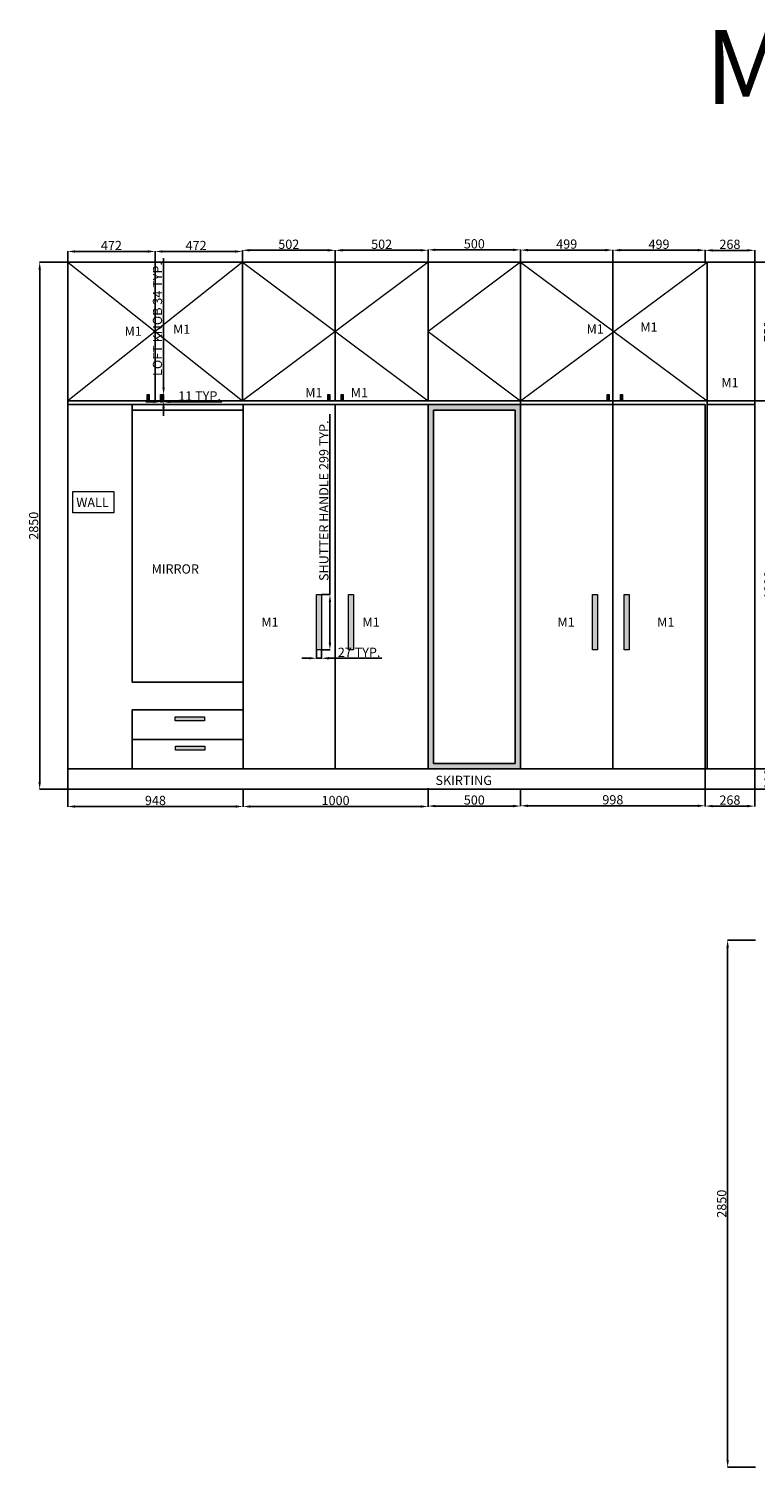
# Model space of a CAD drawing. Units: millimetres. Extents: x 46070 to 59439, y 6883 to 14761.
# Tile 1 of 5: x 46070 to 49997, y 6983 to 14761. Entities that reach past the tile are written whole.
import ezdxf

# ---------------------------------------------------------------- set-up
doc = ezdxf.new("R2010")
doc.units = ezdxf.units.MM
for name, color, linetype, lineweight in [('A-ANNO-DIMS', 2, 'Continuous', 18), ('A-ANNO-TEXT', 7, 'Continuous', 18), ('A-ELEV', 7, 'Continuous', 25), ('A-ELEV-OPEN', 1, 'Continuous', 13), ('A-ELEV-PATT', 8, 'Continuous', 13), ('A-FURN-HDWR', 4, 'Continuous', 18)]:
    doc.layers.add(name, color=color, linetype=linetype, lineweight=lineweight)
doc.styles.get("Standard").update_dxf_attribs({"font": 'arial.ttf'})
doc.dimstyles.new('ISO-25', dxfattribs={"dimtxt": 50, "dimasz": 40, "dimexe": 1.25, "dimexo": 0.625, "dimtad": 1, "dimtxsty": 'Standard', "dimcen": 2.5, "dimadec": 0, "dimazin": 0, "dimtfac": 1, "dimtmove": 0, "dimatfit": 3, "dimfxl": 1, "dimarcsym": 0})

# ---------------------------------------------------------------- blocks, each defined once
blk = doc.blocks.new('*D1')
at = {"layer": 'A-ANNO-DIMS', "color": 0, "lineweight": -2, "transparency": 16777216}
for p, q in [((49995.3, 10759), (50105.5, 10759)), ((50104.2, 10689), (50104.2, 10719)), ((49995.3, 10649), (50105.5, 10649))]:
    blk.add_line(p, q, dxfattribs=at)
at = {"layer": 'A-ANNO-DIMS', "color": 0, "transparency": 16777216}
for points in [[(50097.5, 10719), (50110.9, 10719), (50104.2, 10759)], [(50097.5, 10689), (50110.9, 10689), (50104.2, 10649)]]:
    blk.add_solid(points, dxfattribs=at)
at = {"layer": 'Defpoints', "color": 0, "transparency": 16777216}
for p in [(49994.7, 10759), (50104.2, 10759), (49994.7, 10649)]:
    blk.add_point(p, dxfattribs=at)
at = {"layer": 'A-ANNO-DIMS', "color": 0, "transparency": 16777216, "insert": (50078.1, 10703.9), "char_height": 50, "attachment_point": 5, "rotation": 90}
blk.add_mtext('110', dxfattribs=at)
blk = doc.blocks.new('*D2')
at = {"layer": 'A-ANNO-DIMS', "color": 0, "lineweight": -2, "transparency": 16777216}
for p, q in [((49995.3, 12749), (50105.3, 12749)), ((50104.1, 10799), (50104.1, 12709)), ((49995.3, 10759), (50105.3, 10759))]:
    blk.add_line(p, q, dxfattribs=at)
at = {"layer": 'A-ANNO-DIMS', "color": 0, "transparency": 16777216}
for points in [[(50097.4, 12709), (50110.8, 12709), (50104.1, 12749)], [(50097.4, 10799), (50110.8, 10799), (50104.1, 10759)]]:
    blk.add_solid(points, dxfattribs=at)
at = {"layer": 'Defpoints', "color": 0, "transparency": 16777216}
for p in [(49994.7, 12749), (50104.1, 12749), (49994.7, 10759)]:
    blk.add_point(p, dxfattribs=at)
at = {"layer": 'A-ANNO-DIMS', "color": 0, "transparency": 16777216, "insert": (50077.9, 11754), "char_height": 50, "attachment_point": 5, "rotation": 90}
blk.add_mtext('1990', dxfattribs=at)
blk = doc.blocks.new('*D3')
at = {"layer": 'A-ANNO-DIMS', "color": 0, "lineweight": -2, "transparency": 16777216}
for p, q in [((49995.3, 13499), (50103.6, 13499)), ((50102.3, 12789), (50102.3, 13459)), ((49995.3, 12749), (50103.6, 12749))]:
    blk.add_line(p, q, dxfattribs=at)
at = {"layer": 'A-ANNO-DIMS', "color": 0, "transparency": 16777216}
for points in [[(50095.6, 13459), (50109, 13459), (50102.3, 13499)], [(50095.6, 12789), (50109, 12789), (50102.3, 12749)]]:
    blk.add_solid(points, dxfattribs=at)
at = {"layer": 'Defpoints', "color": 0, "transparency": 16777216}
for p in [(49994.7, 13499), (50102.3, 13499), (49994.7, 12749)]:
    blk.add_point(p, dxfattribs=at)
at = {"layer": 'A-ANNO-DIMS', "color": 0, "transparency": 16777216, "insert": (50076.2, 13124), "char_height": 50, "attachment_point": 5, "rotation": 90}
blk.add_mtext('750', dxfattribs=at)
blk = doc.blocks.new('*D4')
at = {"layer": 'A-ANNO-DIMS', "color": 0, "lineweight": -2, "transparency": 16777216}
for p, q in [((48728.7, 13499.7), (48728.7, 13565.8)), ((49187.7, 13564.6), (48768.7, 13564.6)), ((49227.7, 13499.7), (49227.7, 13565.8))]:
    blk.add_line(p, q, dxfattribs=at)
at = {"layer": 'A-ANNO-DIMS', "color": 0, "transparency": 16777216}
for points in [[(48768.7, 13571.2), (48768.7, 13557.9), (48728.7, 13564.6)], [(49187.7, 13571.2), (49187.7, 13557.9), (49227.7, 13564.6)]]:
    blk.add_solid(points, dxfattribs=at)
at = {"layer": 'Defpoints', "color": 0, "transparency": 16777216}
for p in [(48728.7, 13564.6), (48728.7, 13499), (49227.7, 13499)]:
    blk.add_point(p, dxfattribs=at)
at = {"layer": 'A-ANNO-DIMS', "color": 0, "transparency": 16777216, "insert": (48978.2, 13590.7), "char_height": 50, "attachment_point": 5}
blk.add_mtext('499', dxfattribs=at)
blk = doc.blocks.new('*D5')
at = {"layer": 'A-ANNO-DIMS', "color": 0, "lineweight": -2, "transparency": 16777216}
for p, q in [((49227.7, 13499.7), (49227.7, 13565.1)), ((49267.7, 13563.9), (49686.7, 13563.9)), ((49726.7, 13499.7), (49726.7, 13565.1))]:
    blk.add_line(p, q, dxfattribs=at)
at = {"layer": 'A-ANNO-DIMS', "color": 0, "transparency": 16777216}
for points in [[(49267.7, 13570.6), (49267.7, 13557.2), (49227.7, 13563.9)], [(49686.7, 13570.6), (49686.7, 13557.2), (49726.7, 13563.9)]]:
    blk.add_solid(points, dxfattribs=at)
at = {"layer": 'Defpoints', "color": 0, "transparency": 16777216}
for p in [(49726.7, 13563.9), (49227.7, 13499), (49726.7, 13499)]:
    blk.add_point(p, dxfattribs=at)
at = {"layer": 'A-ANNO-DIMS', "color": 0, "transparency": 16777216, "insert": (49477.2, 13590), "char_height": 50, "attachment_point": 5}
blk.add_mtext('499', dxfattribs=at)
blk = doc.blocks.new('*D6')
at = {"layer": 'A-ANNO-DIMS', "color": 0, "lineweight": -2, "transparency": 16777216}
for p, q in [((48728.7, 10648.4), (48728.7, 10558.4)), ((49726.7, 10648.4), (49726.7, 10558.4)), ((49686.7, 10559.6), (48768.7, 10559.6))]:
    blk.add_line(p, q, dxfattribs=at)
at = {"layer": 'A-ANNO-DIMS', "color": 0, "transparency": 16777216}
for points in [[(48768.7, 10566.3), (48768.7, 10552.9), (48728.7, 10559.6)], [(49686.7, 10566.3), (49686.7, 10552.9), (49726.7, 10559.6)]]:
    blk.add_solid(points, dxfattribs=at)
at = {"layer": 'Defpoints', "color": 0, "transparency": 16777216}
for p in [(48728.7, 10649), (49726.7, 10649), (48728.7, 10559.6)]:
    blk.add_point(p, dxfattribs=at)
at = {"layer": 'A-ANNO-DIMS', "color": 0, "transparency": 16777216, "insert": (49227.7, 10585.8), "char_height": 50, "attachment_point": 5}
blk.add_mtext('998', dxfattribs=at)
blk = doc.blocks.new('*D7')
at = {"layer": 'A-ANNO-DIMS', "color": 0, "lineweight": -2, "transparency": 16777216}
for p, q in [((48228.7, 10648.4), (48228.7, 10557.1)), ((48728.7, 10648.4), (48728.7, 10557.1)), ((48268.7, 10558.4), (48688.7, 10558.4))]:
    blk.add_line(p, q, dxfattribs=at)
at = {"layer": 'A-ANNO-DIMS', "color": 0, "transparency": 16777216}
for points in [[(48268.7, 10565), (48268.7, 10551.7), (48228.7, 10558.4)], [(48688.7, 10565), (48688.7, 10551.7), (48728.7, 10558.4)]]:
    blk.add_solid(points, dxfattribs=at)
at = {"layer": 'Defpoints', "color": 0, "transparency": 16777216}
for p in [(48228.7, 10649), (48728.7, 10649), (48728.7, 10558.4)]:
    blk.add_point(p, dxfattribs=at)
at = {"layer": 'A-ANNO-DIMS', "color": 0, "transparency": 16777216, "insert": (48478.7, 10584.5), "char_height": 50, "attachment_point": 5}
blk.add_mtext('500', dxfattribs=at)
blk = doc.blocks.new('*D8')
at = {"layer": 'A-ANNO-DIMS', "color": 0, "lineweight": -2, "transparency": 16777216}
for p, q in [((48228.7, 13499.7), (48228.7, 13567.1)), ((48268.7, 13565.8), (48688.7, 13565.8)), ((48728.7, 13499.7), (48728.7, 13567.1))]:
    blk.add_line(p, q, dxfattribs=at)
at = {"layer": 'A-ANNO-DIMS', "color": 0, "transparency": 16777216}
for points in [[(48268.7, 13572.5), (48268.7, 13559.2), (48228.7, 13565.8)], [(48688.7, 13572.5), (48688.7, 13559.2), (48728.7, 13565.8)]]:
    blk.add_solid(points, dxfattribs=at)
at = {"layer": 'Defpoints', "color": 0, "transparency": 16777216}
for p in [(48728.7, 13565.8), (48228.7, 13499), (48728.7, 13499)]:
    blk.add_point(p, dxfattribs=at)
at = {"layer": 'A-ANNO-DIMS', "color": 0, "transparency": 16777216, "insert": (48478.7, 13592), "char_height": 50, "attachment_point": 5}
blk.add_mtext('500', dxfattribs=at)
blk = doc.blocks.new('*D9')
at = {"layer": 'A-ANNO-DIMS', "color": 0, "lineweight": -2, "transparency": 16777216}
for p, q in [((47726.7, 13499.7), (47726.7, 13564.7)), ((48188.7, 13563.5), (47766.7, 13563.5)), ((48228.7, 13499.7), (48228.7, 13564.7))]:
    blk.add_line(p, q, dxfattribs=at)
at = {"layer": 'A-ANNO-DIMS', "color": 0, "transparency": 16777216}
for points in [[(47766.7, 13570.2), (47766.7, 13556.8), (47726.7, 13563.5)], [(48188.7, 13570.2), (48188.7, 13556.8), (48228.7, 13563.5)]]:
    blk.add_solid(points, dxfattribs=at)
at = {"layer": 'Defpoints', "color": 0, "transparency": 16777216}
for p in [(47726.7, 13563.5), (47726.7, 13499), (48228.7, 13499)]:
    blk.add_point(p, dxfattribs=at)
at = {"layer": 'A-ANNO-DIMS', "color": 0, "transparency": 16777216, "insert": (47977.7, 13589.7), "char_height": 50, "attachment_point": 5}
blk.add_mtext('502', dxfattribs=at)
blk = doc.blocks.new('*D10')
at = {"layer": 'A-ANNO-DIMS', "color": 0, "lineweight": -2, "transparency": 16777216}
for p, q in [((46752.7, 13499.7), (46752.7, 13558.3)), ((47184.7, 13557.1), (46792.7, 13557.1)), ((47224.7, 13499.7), (47224.7, 13558.3))]:
    blk.add_line(p, q, dxfattribs=at)
at = {"layer": 'A-ANNO-DIMS', "color": 0, "transparency": 16777216}
for points in [[(46792.7, 13563.7), (46792.7, 13550.4), (46752.7, 13557.1)], [(47184.7, 13563.7), (47184.7, 13550.4), (47224.7, 13557.1)]]:
    blk.add_solid(points, dxfattribs=at)
at = {"layer": 'Defpoints', "color": 0, "transparency": 16777216}
for p in [(46752.7, 13557.1), (46752.7, 13499), (47224.7, 13499)]:
    blk.add_point(p, dxfattribs=at)
at = {"layer": 'A-ANNO-DIMS', "color": 0, "transparency": 16777216, "insert": (46974.5, 13582.8), "char_height": 50, "attachment_point": 5}
blk.add_mtext('472', dxfattribs=at)
blk = doc.blocks.new('*D11')
at = {"layer": 'A-ANNO-DIMS', "color": 0, "lineweight": -2, "transparency": 16777216}
for p, q in [((47224.7, 13499.7), (47224.7, 13564.7)), ((47264.7, 13563.5), (47686.7, 13563.5)), ((47726.7, 13499.7), (47726.7, 13564.7))]:
    blk.add_line(p, q, dxfattribs=at)
at = {"layer": 'A-ANNO-DIMS', "color": 0, "transparency": 16777216}
for points in [[(47264.7, 13570.2), (47264.7, 13556.8), (47224.7, 13563.5)], [(47686.7, 13570.2), (47686.7, 13556.8), (47726.7, 13563.5)]]:
    blk.add_solid(points, dxfattribs=at)
at = {"layer": 'Defpoints', "color": 0, "transparency": 16777216}
for p in [(47726.7, 13563.5), (47224.7, 13499), (47726.7, 13499)]:
    blk.add_point(p, dxfattribs=at)
at = {"layer": 'A-ANNO-DIMS', "color": 0, "transparency": 16777216, "insert": (47475.7, 13589.7), "char_height": 50, "attachment_point": 5}
blk.add_mtext('502', dxfattribs=at)
blk = doc.blocks.new('*D12')
at = {"layer": 'A-ANNO-DIMS', "color": 0, "lineweight": -2, "transparency": 16777216}
for p, q in [((46280.7, 13499.7), (46280.7, 13558.4)), ((46320.7, 13557.1), (46712.7, 13557.1)), ((46752.7, 13499.7), (46752.7, 13558.4))]:
    blk.add_line(p, q, dxfattribs=at)
at = {"layer": 'A-ANNO-DIMS', "color": 0, "transparency": 16777216}
for points in [[(46320.7, 13563.8), (46320.7, 13550.4), (46280.7, 13557.1)], [(46712.7, 13563.8), (46712.7, 13550.4), (46752.7, 13557.1)]]:
    blk.add_solid(points, dxfattribs=at)
at = {"layer": 'Defpoints', "color": 0, "transparency": 16777216}
for p in [(46752.7, 13557.1), (46280.7, 13499), (46752.7, 13499)]:
    blk.add_point(p, dxfattribs=at)
at = {"layer": 'A-ANNO-DIMS', "color": 0, "transparency": 16777216, "insert": (46516.7, 13582.8), "char_height": 50, "attachment_point": 5}
blk.add_mtext('472', dxfattribs=at)
blk = doc.blocks.new('*D13')
at = {"layer": 'A-ANNO-DIMS', "color": 0, "lineweight": -2, "transparency": 16777216}
for p, q in [((49726.7, 13499.7), (49726.7, 13564.4)), ((49954.7, 13563.2), (49766.7, 13563.2)), ((49994.7, 13499.7), (49994.7, 13564.4))]:
    blk.add_line(p, q, dxfattribs=at)
at = {"layer": 'A-ANNO-DIMS', "color": 0, "transparency": 16777216}
for points in [[(49766.7, 13569.8), (49766.7, 13556.5), (49726.7, 13563.2)], [(49954.7, 13569.8), (49954.7, 13556.5), (49994.7, 13563.2)]]:
    blk.add_solid(points, dxfattribs=at)
at = {"layer": 'Defpoints', "color": 0, "transparency": 16777216}
for p in [(49726.7, 13563.2), (49726.7, 13499), (49994.7, 13499)]:
    blk.add_point(p, dxfattribs=at)
at = {"layer": 'A-ANNO-DIMS', "color": 0, "transparency": 16777216, "insert": (49860.7, 13589.3), "char_height": 50, "attachment_point": 5}
blk.add_mtext('268', dxfattribs=at)
blk = doc.blocks.new('*D14')
at = {"layer": 'A-ANNO-DIMS', "color": 0, "lineweight": -2, "transparency": 16777216}
for p, q in [((47228.7, 10648.4), (47228.7, 10554.6)), ((48228.7, 10655.9), (48228.7, 10554.6)), ((48188.7, 10555.9), (47268.7, 10555.9))]:
    blk.add_line(p, q, dxfattribs=at)
at = {"layer": 'A-ANNO-DIMS', "color": 0, "transparency": 16777216}
for points in [[(47268.7, 10562.5), (47268.7, 10549.2), (47228.7, 10555.9)], [(48188.7, 10562.5), (48188.7, 10549.2), (48228.7, 10555.9)]]:
    blk.add_solid(points, dxfattribs=at)
at = {"layer": 'Defpoints', "color": 0, "transparency": 16777216}
for p in [(48228.7, 10656.5), (47228.7, 10649), (47228.7, 10555.9)]:
    blk.add_point(p, dxfattribs=at)
at = {"layer": 'A-ANNO-DIMS', "color": 0, "transparency": 16777216, "insert": (47728.7, 10582), "char_height": 50, "attachment_point": 5}
blk.add_mtext('1000', dxfattribs=at)
blk = doc.blocks.new('*D15')
at = {"layer": 'A-ANNO-DIMS', "color": 0, "lineweight": -2, "transparency": 16777216}
for p, q in [((46280.7, 10648.4), (46280.7, 10554.7)), ((47228.7, 10648.4), (47228.7, 10554.7)), ((47188.7, 10555.9), (46320.7, 10555.9))]:
    blk.add_line(p, q, dxfattribs=at)
at = {"layer": 'A-ANNO-DIMS', "color": 0, "transparency": 16777216}
for points in [[(46320.7, 10562.6), (46320.7, 10549.3), (46280.7, 10555.9)], [(47188.7, 10562.6), (47188.7, 10549.3), (47228.7, 10555.9)]]:
    blk.add_solid(points, dxfattribs=at)
at = {"layer": 'Defpoints', "color": 0, "transparency": 16777216}
for p in [(46280.7, 10649), (47228.7, 10649), (46280.7, 10555.9)]:
    blk.add_point(p, dxfattribs=at)
at = {"layer": 'A-ANNO-DIMS', "color": 0, "transparency": 16777216, "insert": (46754.7, 10582.1), "char_height": 50, "attachment_point": 5}
blk.add_mtext('948', dxfattribs=at)
blk = doc.blocks.new('*D16')
at = {"layer": 'A-ANNO-DIMS', "color": 0, "lineweight": -2, "transparency": 16777216}
for p, q in [((49726.7, 10758.4), (49726.7, 10556.8)), ((49994.7, 10758.4), (49994.7, 10556.8)), ((49766.7, 10558.1), (49954.7, 10558.1))]:
    blk.add_line(p, q, dxfattribs=at)
at = {"layer": 'A-ANNO-DIMS', "color": 0, "transparency": 16777216}
for points in [[(49766.7, 10564.7), (49766.7, 10551.4), (49726.7, 10558.1)], [(49954.7, 10564.7), (49954.7, 10551.4), (49994.7, 10558.1)]]:
    blk.add_solid(points, dxfattribs=at)
at = {"layer": 'Defpoints', "color": 0, "transparency": 16777216}
for p in [(49726.7, 10759), (49994.7, 10759), (49994.7, 10558.1)]:
    blk.add_point(p, dxfattribs=at)
at = {"layer": 'A-ANNO-DIMS', "color": 0, "transparency": 16777216, "insert": (49860.7, 10584.2), "char_height": 50, "attachment_point": 5}
blk.add_mtext('268', dxfattribs=at)
blk = doc.blocks.new('*D17')
at = {"layer": 'A-ANNO-DIMS', "color": 0, "lineweight": -2, "transparency": 16777216}
for p, q in [((46280.1, 13499), (46127.7, 13499)), ((46129, 10689), (46129, 13459)), ((46280.1, 10649), (46127.7, 10649))]:
    blk.add_line(p, q, dxfattribs=at)
at = {"layer": 'A-ANNO-DIMS', "color": 0, "transparency": 16777216}
for points in [[(46122.3, 13459), (46135.6, 13459), (46129, 13499)], [(46122.3, 10689), (46135.6, 10689), (46129, 10649)]]:
    blk.add_solid(points, dxfattribs=at)
at = {"layer": 'Defpoints', "color": 0, "transparency": 16777216}
for p in [(46129, 13499), (46280.7, 13499), (46280.7, 10649)]:
    blk.add_point(p, dxfattribs=at)
at = {"layer": 'A-ANNO-DIMS', "color": 0, "transparency": 16777216, "insert": (46102.8, 12074), "char_height": 50, "attachment_point": 5, "rotation": 90}
blk.add_mtext('2850', dxfattribs=at)
blk = doc.blocks.new('*D96')
at = {"layer": 'A-ANNO-DIMS', "color": 0, "lineweight": -2, "transparency": 16777216}
for p, q in [((49999.5, 9833.2), (49847.1, 9833.2)), ((49848.4, 7023.2), (49848.4, 9793.2)), ((49999.5, 6983.2), (49847.1, 6983.2))]:
    blk.add_line(p, q, dxfattribs=at)
at = {"layer": 'A-ANNO-DIMS', "color": 0, "transparency": 16777216}
for points in [[(49841.7, 9793.2), (49855, 9793.2), (49848.4, 9833.2)], [(49841.7, 7023.2), (49855, 7023.2), (49848.4, 6983.2)]]:
    blk.add_solid(points, dxfattribs=at)
at = {"layer": 'Defpoints', "color": 0, "transparency": 16777216}
for p in [(49848.4, 9833.2), (50000.1, 9833.2), (50000.1, 6983.2)]:
    blk.add_point(p, dxfattribs=at)
at = {"layer": 'A-ANNO-DIMS', "color": 0, "transparency": 16777216, "insert": (49822.2, 8408.2), "char_height": 50, "attachment_point": 5, "rotation": 90}
blk.add_mtext('2850', dxfattribs=at)
blk = doc.blocks.new('HANDLE-BAR-300')
blk.add_lwpolyline([(0, 299.3), (26.9, 299.3), (26.9, 0), (0, 0)], close=True)
blk = doc.blocks.new('DRAWER-PULL-160')
blk.add_lwpolyline([(0, 22.3), (158.3, 22.3), (158.3, 0), (0, 0)], close=True)
blk = doc.blocks.new('LOFT-KNOB')
blk.add_lwpolyline([(0, 33.9), (11, 33.9), (11, 0), (0, 0)], close=True)
blk = doc.blocks.new('*D100')
at = {"layer": 'A-ANNO-DIMS', "color": 0, "lineweight": -2, "transparency": 16777216}
for p, q in [((47698.1, 11701.7), (47698.1, 12677)), ((47653.9, 11701.7), (47699.4, 11701.7)), ((47698.1, 11442.5), (47698.1, 11661.7)), ((47653.9, 11402.5), (47699.4, 11402.5))]:
    blk.add_line(p, q, dxfattribs=at)
at = {"layer": 'A-ANNO-DIMS', "color": 0, "transparency": 16777216}
for points in [[(47691.5, 11661.7), (47704.8, 11661.7), (47698.1, 11701.7)], [(47691.5, 11442.5), (47704.8, 11442.5), (47698.1, 11402.5)]]:
    blk.add_solid(points, dxfattribs=at)
at = {"layer": 'Defpoints', "color": 0, "transparency": 16777216}
for p in [(47653.2, 11701.7), (47698.1, 11701.7), (47653.2, 11402.5)]:
    blk.add_point(p, dxfattribs=at)
at = {"layer": 'A-ANNO-DIMS', "color": 0, "transparency": 16777216, "insert": (47671.7, 12209.4), "char_height": 50, "attachment_point": 5, "rotation": 90}
blk.add_mtext('SHUTTER HANDLE 299 TYP.', dxfattribs=at)
blk = doc.blocks.new('*D101')
at = {"layer": 'A-ANNO-DIMS', "color": 0, "lineweight": -2, "transparency": 16777216}
for p, q in [((47586.3, 11357.6), (47546.3, 11357.6)), ((47626.3, 11401.8), (47626.3, 11356.3)), ((47626.3, 11357.6), (47653.2, 11357.6)), ((47653.2, 11401.8), (47653.2, 11356.3)), ((47693.2, 11357.6), (47978.7, 11357.6))]:
    blk.add_line(p, q, dxfattribs=at)
at = {"layer": 'A-ANNO-DIMS', "color": 0, "transparency": 16777216}
for points in [[(47586.3, 11364.2), (47586.3, 11350.9), (47626.3, 11357.6)], [(47693.2, 11364.2), (47693.2, 11350.9), (47653.2, 11357.6)]]:
    blk.add_solid(points, dxfattribs=at)
at = {"layer": 'Defpoints', "color": 0, "transparency": 16777216}
for p in [(47626.3, 11402.5), (47653.2, 11402.5), (47653.2, 11357.6)]:
    blk.add_point(p, dxfattribs=at)
at = {"layer": 'A-ANNO-DIMS', "color": 0, "transparency": 16777216, "insert": (47856, 11383.3), "char_height": 50, "attachment_point": 5}
blk.add_mtext('27 TYP.', dxfattribs=at)
blk = doc.blocks.new('*D102')
at = {"layer": 'A-ANNO-DIMS', "color": 0, "lineweight": -2, "transparency": 16777216}
for p, q in [((46798.7, 12822.9), (46798.7, 13520.6)), ((46794.2, 12782.9), (46799.9, 12782.9)), ((46798.7, 12749), (46798.7, 12782.9)), ((46794.2, 12749), (46799.9, 12749)), ((46798.7, 12709), (46798.7, 12669))]:
    blk.add_line(p, q, dxfattribs=at)
at = {"layer": 'A-ANNO-DIMS', "color": 0, "transparency": 16777216}
for points in [[(46792, 12822.9), (46805.3, 12822.9), (46798.7, 12782.9)], [(46792, 12709), (46805.3, 12709), (46798.7, 12749)]]:
    blk.add_solid(points, dxfattribs=at)
at = {"layer": 'Defpoints', "color": 0, "transparency": 16777216}
for p in [(46793.6, 12782.9), (46798.7, 12782.9), (46793.6, 12749)]:
    blk.add_point(p, dxfattribs=at)
at = {"layer": 'A-ANNO-DIMS', "color": 0, "transparency": 16777216, "insert": (46772.2, 13191.8), "char_height": 50, "attachment_point": 5, "rotation": 90}
blk.add_mtext('LOFT KNOB 34 TYP.', dxfattribs=at)
blk = doc.blocks.new('*D103')
at = {"layer": 'A-ANNO-DIMS', "color": 0, "lineweight": -2, "transparency": 16777216}
for p, q in [((46742.6, 12743.9), (46702.6, 12743.9)), ((46782.6, 12748.4), (46782.6, 12742.7)), ((46782.6, 12743.9), (46793.6, 12743.9)), ((46793.6, 12748.4), (46793.6, 12742.7)), ((46833.6, 12743.9), (47113.5, 12743.9))]:
    blk.add_line(p, q, dxfattribs=at)
at = {"layer": 'A-ANNO-DIMS', "color": 0, "transparency": 16777216}
for points in [[(46742.6, 12750.6), (46742.6, 12737.3), (46782.6, 12743.9)], [(46833.6, 12750.6), (46833.6, 12737.3), (46793.6, 12743.9)]]:
    blk.add_solid(points, dxfattribs=at)
at = {"layer": 'Defpoints', "color": 0, "transparency": 16777216}
for p in [(46782.6, 12749), (46793.6, 12749), (46793.6, 12743.9)]:
    blk.add_point(p, dxfattribs=at)
at = {"layer": 'A-ANNO-DIMS', "color": 0, "transparency": 16777216, "insert": (46993.5, 12769.7), "char_height": 50, "attachment_point": 5}
blk.add_mtext('11 TYP.', dxfattribs=at)

msp = doc.modelspace()

# ---------------------------------------------------------------- hatches: boundary and pattern name
at = {"layer": 'A-ELEV-PATT'}
h = msp.add_hatch(color=256, dxfattribs=at)
h.dxf.hatch_style = 1
h.paths.add_polyline_path([(46710.434, 12749.028), (46721.43, 12749.028), (46721.43, 12782.906), (46710.434, 12782.906)])
h = msp.add_hatch(color=256, dxfattribs=at)
h.dxf.hatch_style = 1
h.paths.add_polyline_path([(46782.587, 12749.028), (46793.583, 12749.028), (46793.583, 12782.906), (46782.587, 12782.906)])
h = msp.add_hatch(color=256, dxfattribs=at)
h.dxf.hatch_style = 1
h.paths.add_polyline_path([(47697.499, 12782.906), (47686.503, 12782.906), (47686.503, 12749.028), (47697.499, 12749.028)])
h = msp.add_hatch(color=256, dxfattribs=at)
h.dxf.hatch_style = 1
h.paths.add_polyline_path([(47769.652, 12782.906), (47758.656, 12782.906), (47758.656, 12749.028), (47769.652, 12749.028)])
h = msp.add_hatch(color=256, dxfattribs=at)
h.dxf.hatch_style = 1
h.paths.add_polyline_path([(49208.449, 12782.906), (49197.453, 12782.906), (49197.453, 12749.028), (49208.449, 12749.028)])
h = msp.add_hatch(color=256, dxfattribs=at)
h.dxf.hatch_style = 1
h.paths.add_polyline_path([(49280.602, 12782.906), (49269.606, 12782.906), (49269.606, 12749.028), (49280.602, 12749.028)])
h = msp.add_hatch(color=256, dxfattribs=at)
h.dxf.hatch_style = 1
h.paths.add_polyline_path([(48728.695, 12729.028), (48228.695, 12729.028), (48228.695, 10759.028), (48728.695, 10759.028)])
h.paths.add_polyline_path([(48698.695, 10789.028), (48258.695, 10789.028), (48258.695, 12699.028), (48698.695, 12699.028)], flags=16)
h = msp.add_hatch(color=256, dxfattribs=at)
h.dxf.hatch_style = 1
h.paths.add_polyline_path([(47798.155, 11402.45), (47825.073, 11402.45), (47825.073, 11701.733), (47798.155, 11701.733)])
h.paths.add_polyline_path([(47626.327, 11402.45), (47653.245, 11402.45), (47653.245, 11701.733), (47626.327, 11701.733)])
h = msp.add_hatch(color=256, dxfattribs=at)
h.dxf.hatch_style = 1
h.paths.add_polyline_path([(49289.261, 11402.45), (49316.18, 11402.45), (49316.18, 11701.733), (49289.261, 11701.733)])
h.paths.add_polyline_path([(49117.434, 11402.45), (49144.352, 11402.45), (49144.352, 11701.733), (49117.434, 11701.733)])
h = msp.add_hatch(color=256, dxfattribs=at)
h.dxf.hatch_style = 1
h.paths.add_polyline_path([(47019.791, 11018.624), (47019.791, 11040.889), (46861.488, 11040.889), (46861.488, 11018.624)])
h.paths.add_polyline_path([(47022.135, 10860.421), (47022.135, 10882.686), (46863.833, 10882.686), (46863.833, 10860.421)])

# ---------------------------------------------------------------- linework, layer by layer
at = {"layer": 'A-ANNO-TEXT'}
msp.add_lwpolyline([(46307.816, 12259.951), (46529.722, 12259.951), (46529.722, 12143.105), (46307.816, 12143.105)], close=True, dxfattribs=at)
at = {"layer": 'A-ELEV'}
for p, q in [((49994.695, 13499.028), (46280.695, 13499.028)), ((46280.695, 10649.028), (46280.695, 13499.028)), ((46752.695, 12749.028), (46752.695, 13499.028)), ((47224.695, 12749.028), (47224.695, 13499.028)), ((47726.695, 12749.028), (47726.695, 13499.028)), ((48228.695, 12749.028), (48228.695, 13499.028)), ((48728.695, 10759.028), (48728.695, 13499.028)), ((49227.695, 12729.028), (49227.695, 13499.028)), ((49736.695, 10759.028), (49736.695, 13499.028)), ((49994.695, 10649.028), (49994.695, 13499.028)), ((49994.695, 12749.028), (46280.695, 12749.028)), ((49726.695, 12729.028), (46280.695, 12729.028)), ((46628.695, 11229.028), (46628.695, 12729.028)), ((47228.695, 12699.028), (46628.695, 12699.028)), ((47228.695, 10759.028), (47228.695, 12729.028)), ((47726.695, 12729.028), (47726.695, 10759.028)), ((48228.695, 10759.028), (48228.695, 12729.028)), ((48258.695, 10789.028), (48258.695, 12699.028)), ((48698.695, 12699.028), (48258.695, 12699.028)), ((48698.695, 10789.028), (48698.695, 12699.028)), ((49227.695, 10759.028), (49227.695, 12729.028)), ((49726.695, 10759.028), (49726.695, 12729.028)), ((49994.695, 12729.028), (49736.695, 12729.028)), ((47228.695, 11229.028), (46628.695, 11229.028)), ((46628.695, 10759.028), (46628.695, 11079.028)), ((47228.695, 11079.028), (46628.695, 11079.028)), ((47228.695, 10919.028), (46628.695, 10919.028)), ((49994.695, 10759.028), (46280.695, 10759.028)), ((48698.695, 10789.028), (48258.695, 10789.028)), ((46280.695, 10649.028), (49994.695, 10649.028))]:
    msp.add_line(p, q, dxfattribs=at)
at = {"layer": 'A-ELEV-OPEN'}
for p, q in [((46280.695, 13499.028), (47224.695, 12749.028)), ((47224.695, 13499.028), (46280.695, 12749.028)), ((47224.695, 13499.028), (48228.695, 12749.028)), ((48228.695, 13499.028), (47224.695, 12749.028)), ((48728.695, 13499.028), (48228.695, 13124.028)), ((48728.695, 13499.028), (49736.695, 12749.028)), ((48728.695, 12749.028), (49736.695, 13499.028)), ((48228.695, 13124.028), (48728.695, 12749.028))]:
    msp.add_line(p, q, dxfattribs=at)

# ---------------------------------------------------------------- block references
at = {"layer": 'A-FURN-HDWR'}
for name, p in [('LOFT-KNOB', (46710.434, 12749.028)), ('LOFT-KNOB', (46782.587, 12749.028)), ('LOFT-KNOB', (47686.503, 12749.028)), ('LOFT-KNOB', (47758.656, 12749.028)), ('LOFT-KNOB', (49197.453, 12749.028)), ('LOFT-KNOB', (49269.606, 12749.028)), ('HANDLE-BAR-300', (47626.327, 11402.45)), ('HANDLE-BAR-300', (47798.154, 11402.45)), ('HANDLE-BAR-300', (49117.434, 11402.45)), ('HANDLE-BAR-300', (49289.261, 11402.45)), ('DRAWER-PULL-160', (46861.488, 11018.625)), ('DRAWER-PULL-160', (46863.833, 10860.421))]:
    msp.add_blockref(name, p, dxfattribs=at)

# ---------------------------------------------------------------- texts
at = {"layer": 'A-ANNO-TEXT', "attachment_point": 1}
for s, width, insert, char_height in [('MBR WARDROBE ELEVATION', 11748.56084, (49726.408, 14754.198), 400), ('M1', 502.17574, (46587.938, 13150.982), 50), ('M1', 502.17574, (46850.048, 13161.796), 50), ('M1', 502.17574, (49085.653, 13163.409), 50), ('M1', 502.17574, (49376.159, 13173.251), 50), ('M1', 502.17574, (49814.377, 12873.082), 50), ('M1', 502.17574, (47564.737, 12818.972), 50), ('M1', 502.17574, (47810.977, 12818.354), 50), ('WALL', 502.17574, (46326.904, 12225.049), 50), ('MIRROR', 502.17574, (46733.9, 11865.46), 50), ('M1', 502.17574, (47327.419, 11577.792), 50), ('M1', 502.17574, (47873.868, 11577.792), 50), ('M1', 502.17574, (48927.985, 11577.792), 50), ('M1', 502.17574, (49467.195, 11577.792), 50), ('SKIRTING ', 502.17574, (48268.828, 10722.155), 50)]:
    msp.add_mtext_dynamic_manual_height_columns(s, width=width, gutter_width=12.5, heights=[0], dxfattribs=dict(at, insert=insert, char_height=char_height))

# ---------------------------------------------------------------- dimensions: what is measured, and where the dimension line sits
at = {"layer": 'A-ANNO-DIMS'}
for base, p1, p2, picture, middle in [((46752.695, 13557.108), (46280.695, 13499.028), (46752.695, 13499.028), '*D12', (46516.695, 13582.835)), ((47726.695, 13563.499), (47224.695, 13499.028), (47726.695, 13499.028), '*D11', (47475.695, 13589.653)), ((47726.695, 13563.499), (48228.695, 13499.028), (47726.695, 13499.028), '*D9', (47977.695, 13589.653)), ((48728.695, 13565.827), (48228.695, 13499.028), (48728.695, 13499.028), '*D8', (48478.695, 13591.981)), ((48728.695, 13564.577), (49227.695, 13499.028), (48728.695, 13499.028), '*D4', (48978.195, 13590.731)), ((49726.695, 13563.885), (49227.695, 13499.028), (49726.695, 13499.028), '*D5', (49477.195, 13590.038)), ((49726.695, 13563.165), (49994.695, 13499.028), (49726.695, 13499.028), '*D13', (49860.695, 13589.319)), ((49994.695, 10558.068), (49726.695, 10759.028), (49994.695, 10759.028), '*D16', (49860.695, 10584.221)), ((47228.695, 10555.852), (48228.695, 10656.503), (47228.695, 10649.028), '*D14', (47728.695, 10582.005)), ((46280.695, 10555.941), (47228.695, 10649.028), (46280.695, 10649.028), '*D15', (46754.695, 10582.095)), ((48728.695, 10558.365), (48228.695, 10649.028), (48728.695, 10649.028), '*D7', (48478.695, 10584.519)), ((48728.695, 10559.615), (49726.695, 10649.028), (48728.695, 10649.028), '*D6', (49227.695, 10585.769))]:
    dim = msp.add_linear_dim(base=base, p1=p1, p2=p2, dimstyle='ISO-25', override={"dimclrd": 0, "dimclre": 0, "dimclrt": 0}, dxfattribs=at)
    dim.commit()
    dim.dimension.update_dxf_attribs({"geometry": picture, "text_midpoint": middle})
dim = msp.add_linear_dim(base=(46752.695, 13557.074), p1=(47224.695, 13499.028), p2=(46752.695, 13499.028), dimstyle='ISO-25', override={"dimclrd": 0, "dimclre": 0, "dimclrt": 0}, dxfattribs=at)
dim.commit()
dim.dimension.update_dxf_attribs({"geometry": '*D10', "text_midpoint": (46974.548, 13557.074), "dimtype": 160})
for base, p1, p2, picture, middle in [((46128.968, 13499.028), (46280.695, 10649.028), (46280.695, 13499.028), '*D17', (46102.814, 12074.028)), ((50102.311, 13499.028), (49994.695, 12749.028), (49994.695, 13499.028), '*D3', (50076.157, 13124.028)), ((49848.383, 9833.249), (50000.11, 6983.249), (50000.11, 9833.249), '*D96', (49822.229, 8408.249))]:
    dim = msp.add_linear_dim(base=base, p1=p1, p2=p2, angle=90, dimstyle='ISO-25', override={"dimclrd": 0, "dimclre": 0, "dimclrt": 0}, dxfattribs=at)
    dim.commit()
    dim.dimension.update_dxf_attribs({"geometry": picture, "text_midpoint": middle})
for base, p1, p2, text, picture, middle in [((46798.665, 12782.906), (46793.583, 12749.028), (46793.583, 12782.906), 'LOFT KNOB <> TYP.', '*D102', (46772.153, 13191.754)), ((47698.138, 11701.733), (47653.245, 11402.45), (47653.245, 11701.733), 'SHUTTER HANDLE <> TYP.', '*D100', (47671.66, 12209.361))]:
    dim = msp.add_linear_dim(base=base, p1=p1, p2=p2, angle=90, text=text, dimstyle='ISO-25', override={"dimdec": 0, "dimrnd": 0, "dimzin": 0, "dimlunit": 2}, dxfattribs=at)
    dim.commit()
    dim.dimension.update_dxf_attribs({"geometry": picture, "text_midpoint": middle})
for base, p1, p2, picture, middle in [((46793.583, 12743.947), (46782.587, 12749.028), (46793.583, 12749.028), '*D103', (46993.546, 12769.691)), ((47653.245, 11357.558), (47626.327, 11402.45), (47653.245, 11402.45), '*D101', (47855.988, 11383.302))]:
    dim = msp.add_linear_dim(base=base, p1=p1, p2=p2, text='<> TYP.', dimstyle='ISO-25', override={"dimdec": 0, "dimrnd": 0, "dimzin": 0, "dimlunit": 2}, dxfattribs=at)
    dim.commit()
    dim.dimension.update_dxf_attribs({"geometry": picture, "text_midpoint": middle})
for base, p1, p2, picture, middle in [((50104.089, 12749.028), (49994.695, 10759.028), (49994.695, 12749.028), '*D2', (50104.089, 11754.028)), ((50104.213, 10759.028), (49994.695, 10649.028), (49994.695, 10759.028), '*D1', (50104.213, 10703.926))]:
    dim = msp.add_linear_dim(base=base, p1=p1, p2=p2, angle=90, dimstyle='ISO-25', override={"dimclrd": 0, "dimclre": 0, "dimclrt": 0}, dxfattribs=at)
    dim.commit()
    dim.dimension.update_dxf_attribs({"geometry": picture, "text_midpoint": middle, "dimtype": 160})

doc.saveas('drawing.dxf')
